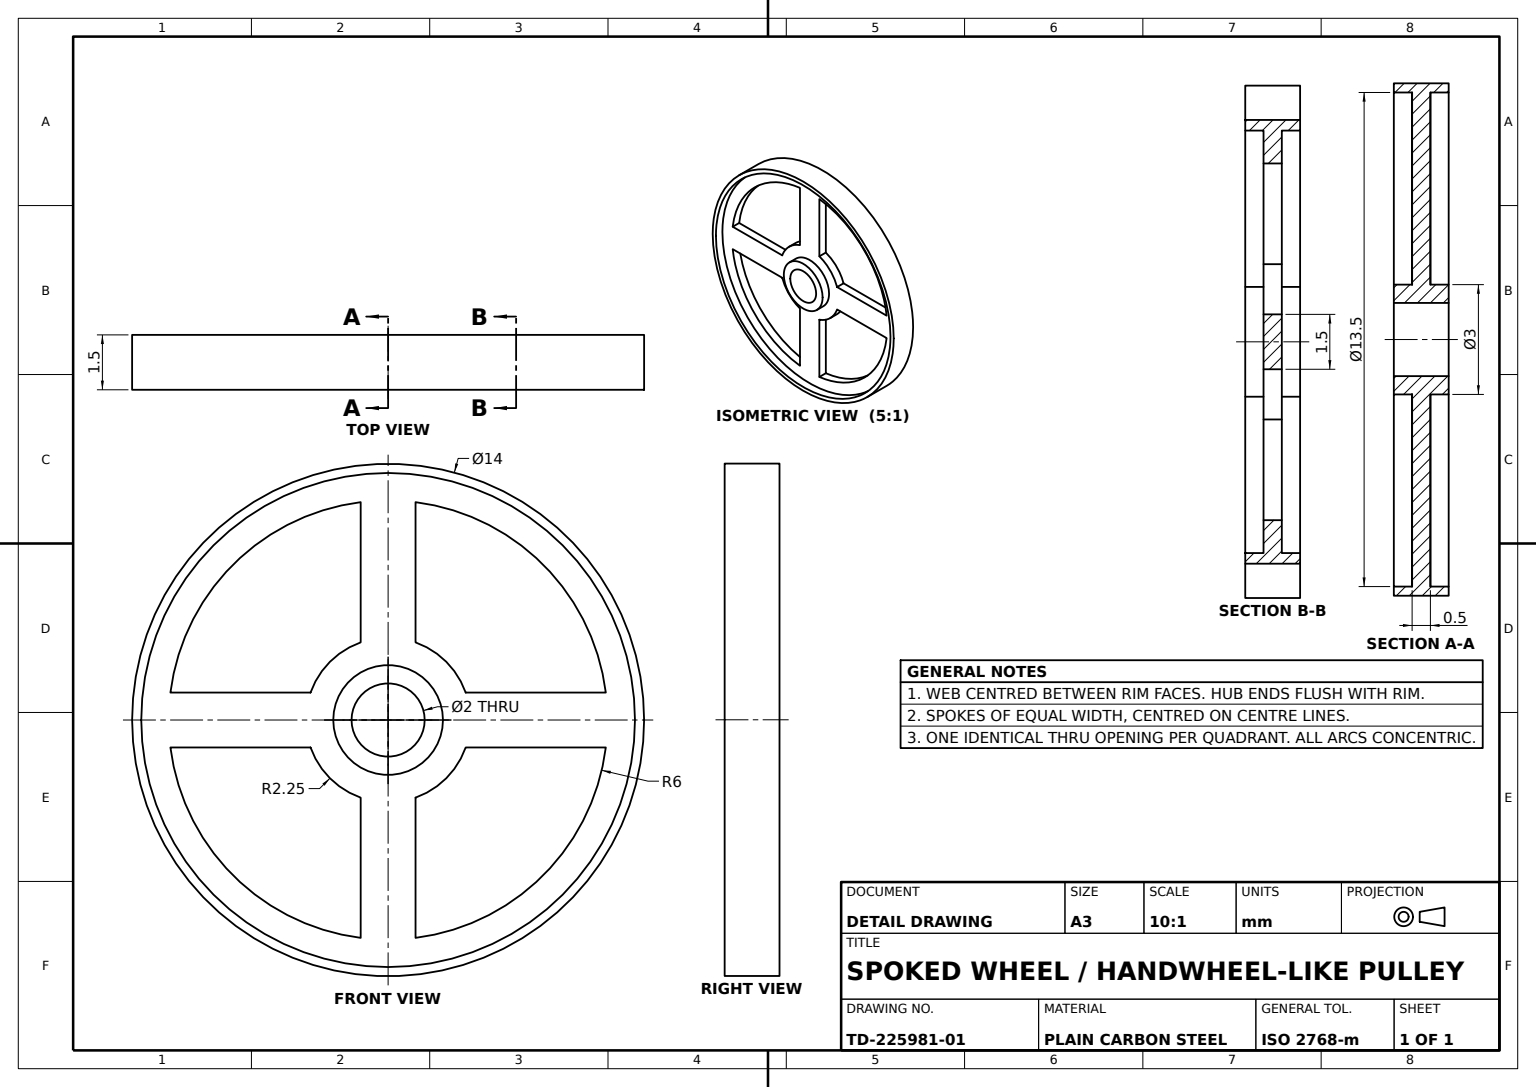
from build123d import *
from build123d.topology import SkipClean

# Parameters (mm, degrees)
HUB_CORE_SKETCH_R           = 2.25
HUB_CORE_DEPTH              = 0.5
HUB_FLANGE_SKETCH_R         = 6
HUB_FLANGE_6_DEPTH          = 0.5
FRONT_HUB_BOSS_SKETCH_R     = 2.25
FRONT_HUB_BOSS_DEPTH        = 0.5
CROSS_START                 = -0.5
CROSS_SLOT_CUT_DEPTH        = 0.5
WEB_START                   = -0.5
WEB_RING_SKETCH_R           = 6.75
WEB_RING_SKETCH_R_2         = 6
WEB_RING_13_5_DEPTH         = 0.5
FRONT_START                 = -0.5
FRONT_HUB_HOLE_SKETCH_R     = 2.25
FRONT_HUB_HOLE_CUT_DEPTH    = 0.5
BACK_HUB_RECESS_SKETCH_R    = 2.25
BACK_HUB_RECESS_CUT_DEPTH   = 0.5
HUB_RING_A_SKETCH_R         = 1.5
HUB_RING_A_DEPTH            = 0.5
HUB_START                   = 0.5
HUB_RING_B_SKETCH_R         = 1.5
HUB_RING_B_DEPTH            = 0.5
SPOKE_1_DEPTH               = 1.5
SPOKE_1_GROOVE_A_DEPTH      = 0.625
SPOKE_1_GROOVE_B_DEPTH      = 0.625
SPOKE_2_DEPTH               = 1.5
SPOKE_3_DEPTH               = 1.5
SPOKE_4_DEPTH               = 1.5
SPOKE_GROOVES_A_DEPTH       = 0.65
SPOKE_GROOVES_B_DEPTH       = 0.65
CROSS_SPOKES_DEPTH          = 1.5
CROSS_SPOKES_2_DEPTH        = 1.5
CROSS_SPOKES_3_DEPTH        = 1.5
CROSS_SPOKES_4_DEPTH        = 1.5
CROSS_SPOKE_GROOVES_A_DEPTH = 0.625
CROSS_SPOKE_GROOVES_B_DEPTH = 0.625
CENTRE_HOLE_SKETCH_R        = 1
CENTRE_HOLE_CUT_DEPTH       = 10
RIM_START                   = -0.5
RIM_RING_1_SKETCH_R         = 7
RIM_RING_1_SKETCH_R_2       = 6.75
RIM_RING_1_14_DEPTH         = 0.5
RIM_RING_2_SKETCH_R         = 7
RIM_RING_2_SKETCH_R_2       = 6.75
RIM_RING_2_14_DEPTH         = 0.5
RIM_START_2                 = 0.5
RIM_RING_3_SKETCH_R         = 7
RIM_RING_3_SKETCH_R_2       = 6.75
RIM_RING_3_14_DEPTH         = 0.5


with BuildPart() as part:
    # Hub Core Sketch → Hub Core (new body)
    with BuildSketch(Plane.XY):
        Circle(HUB_CORE_SKETCH_R)
    extrude(amount=HUB_CORE_DEPTH)

    # Hub Flange Sketch → Hub Flange Ø6 (add)
    with BuildSketch(Plane.XY.offset(0.5)):
        Circle(HUB_FLANGE_SKETCH_R)
    extrude(amount=HUB_FLANGE_6_DEPTH)

    # Front Hub Boss Sketch → Front Hub Boss (add)
    with BuildSketch(Plane.XY.offset(1)):
        Circle(FRONT_HUB_BOSS_SKETCH_R)
    extrude(amount=FRONT_HUB_BOSS_DEPTH)

    # Cross Slot Sketch → Cross Slot Cut (cut)
    with SkipClean():  # the faces are left unmerged after this step: merging them gives an invalid solid
        with BuildSketch(Plane.XY.offset(1).offset(CROSS_START)):
            with BuildLine():
                ThreePointArc((-2.121320344, 0.75), (-1.590990258, 1.590990258), (-0.75, 2.121320344))
                Line((-0.75, 2.121320344), (-0.75, 5.95294045))
                ThreePointArc((-0.75, 5.95294045), (-4.242640687, 4.242640687), (-5.95294045, 0.75))
                Line((-5.95294045, 0.75), (-2.121320344, 0.75))
            make_face()
            with BuildLine():
                Line((0.75, 5.95294045), (0.75, 2.121320344))
                ThreePointArc((0.75, 2.121320344), (1.590990258, 1.590990258), (2.121320344, 0.75))
                Line((2.121320344, 0.75), (5.95294045, 0.75))
                ThreePointArc((5.95294045, 0.75), (4.242640687, 4.242640687), (0.75, 5.95294045))
            make_face()
            with BuildLine():
                ThreePointArc((2.121320344, -0.75), (1.590990258, -1.590990258), (0.75, -2.121320344))
                Line((0.75, -2.121320344), (0.75, -5.95294045))
                ThreePointArc((0.75, -5.95294045), (4.242640687, -4.242640687), (5.95294045, -0.75))
                Line((5.95294045, -0.75), (2.121320344, -0.75))
            make_face()
            with BuildLine():
                Line((-0.75, -5.95294045), (-0.75, -2.121320344))
                ThreePointArc((-0.75, -2.121320344), (-1.590990258, -1.590990258), (-2.121320344, -0.75))
                Line((-2.121320344, -0.75), (-5.95294045, -0.75))
                ThreePointArc((-5.95294045, -0.75), (-4.242640687, -4.242640687), (-0.75, -5.95294045))
            make_face()
        extrude(amount=CROSS_SLOT_CUT_DEPTH, mode=Mode.SUBTRACT)

    # Web Ring Sketch → Web Ring Ø13.5 (add)
    with SkipClean():  # the faces are left unmerged after this step: merging them gives an invalid solid
        with BuildSketch(Plane.XY.offset(1).offset(WEB_START)):
            Circle(WEB_RING_SKETCH_R)
            Circle(WEB_RING_SKETCH_R_2, mode=Mode.SUBTRACT)
        extrude(amount=WEB_RING_13_5_DEPTH)

    # Front Hub Hole Sketch → Front Hub Hole Cut (cut)
    with SkipClean():  # the faces are left unmerged after this step: merging them gives an invalid solid
        with BuildSketch(Plane.XY.offset(1.5).offset(FRONT_START)):
            with Locations(Location((0, 0, 0), (0, 0, 199.471220634))):
                Circle(FRONT_HUB_HOLE_SKETCH_R)
        extrude(amount=FRONT_HUB_HOLE_CUT_DEPTH, mode=Mode.SUBTRACT)

    # Back Hub Recess Sketch → Back Hub Recess Cut (cut)
    with BuildSketch(Plane(origin=(0, 0, 0), x_dir=(-1, 0, 0), z_dir=(0, 0, -1))):
        Circle(BACK_HUB_RECESS_SKETCH_R)
    extrude(amount=-BACK_HUB_RECESS_CUT_DEPTH, mode=Mode.SUBTRACT)

    # Hub Ring A Sketch → Hub Ring A (add)
    with BuildSketch(Plane(origin=(0, 0, 0.5), x_dir=(-1, 0, 0), z_dir=(0, 0, -1))):
        Circle(HUB_RING_A_SKETCH_R)
    extrude(amount=HUB_RING_A_DEPTH)

    # Hub Ring B Sketch → Hub Ring B (add)
    with BuildSketch(Plane.XY.offset(1).offset(HUB_START)):
        with Locations(Location((0, 0, 0), (0, 0, 180))):
            Circle(HUB_RING_B_SKETCH_R)
    extrude(amount=-HUB_RING_B_DEPTH)

    # Centre Hole Sketch → Centre Hole Cut (cut)
    with BuildSketch(Plane.XY.offset(1.5)):
        Circle(CENTRE_HOLE_SKETCH_R)
    extrude(amount=-CENTRE_HOLE_CUT_DEPTH, mode=Mode.SUBTRACT)

    # Rim Ring 1 Sketch → Rim Ring 1 Ø14 (add)
    with BuildSketch(Plane.XY.offset(1).offset(RIM_START)):
        Circle(RIM_RING_1_SKETCH_R)
        Circle(RIM_RING_1_SKETCH_R_2, mode=Mode.SUBTRACT)
    extrude(amount=RIM_RING_1_14_DEPTH)

    # Rim Ring 2 Sketch → Rim Ring 2 Ø14 (add)
    with BuildSketch(Plane.XY.offset(1)):
        Circle(RIM_RING_2_SKETCH_R)
        Circle(RIM_RING_2_SKETCH_R_2, mode=Mode.SUBTRACT)
    extrude(amount=RIM_RING_2_14_DEPTH)

    # Rim Ring 3 Sketch → Rim Ring 3 Ø14 (add)
    with BuildSketch(Plane(origin=(0, 0, 0.5), x_dir=(-1, 0, 0), z_dir=(0, 0, -1)).offset(RIM_START_2)):
        with Locations(Location((0, 0, 0), (0, 0, 180))):
            Circle(RIM_RING_3_SKETCH_R)
        with Locations(Location((0, 0, 0), (0, 0, 180))):
            Circle(RIM_RING_3_SKETCH_R_2, mode=Mode.SUBTRACT)
    extrude(amount=-RIM_RING_3_14_DEPTH)


with BuildPart() as body_2:
    # Spoke 1 Sketch → Spoke 1 (new body)
    with BuildSketch(Plane.XZ.offset(0.75)):
        Polygon((-1.5, 1.5), (-1.5, 1), (-6.75, 1), (-5.25, 1.5), align=None)
    extrude(amount=-SPOKE_1_DEPTH)

    # Spoke 1 Groove A Sketch → Spoke 1 Groove A (cut)
    with BuildSketch(Plane.XZ.offset(0.75)):
        Polygon((-6.75, 1), (-5.25, 1.5), (-1.5, 1.5), (-1.5, 1), align=None)
    extrude(amount=-SPOKE_1_GROOVE_A_DEPTH, mode=Mode.SUBTRACT)

    # Spoke 1 Groove B Sketch → Spoke 1 Groove B (cut)
    with BuildSketch(Plane(origin=(0, 0.75, 0), x_dir=(1, 0, 0), z_dir=(0, 1, 0))):
        Polygon((-1.5, -1.5), (-1.5, -1), (-6.75, -1), (-5.25, -1.5), align=None)
    extrude(amount=-SPOKE_1_GROOVE_B_DEPTH, mode=Mode.SUBTRACT)


with BuildPart() as body_3:
    # Spoke 2 Sketch → Spoke 2 (new body)
    with BuildSketch(Plane.XZ.offset(0.75)):
        Polygon((5.25, 1.5), (1.5, 1.5), (1.5, 1), (2.121320344, 1), (5.95294045, 1), (6.75, 1), align=None)
    extrude(amount=-SPOKE_2_DEPTH)


with BuildPart() as body_4:
    # Spoke 3 Sketch → Spoke 3 (new body)
    with BuildSketch(Plane.XZ.offset(0.75)):
        Polygon((1.5, 0), (1.5, 0.5), (6.75, 0.5), (5.25, 0), align=None)
    extrude(amount=-SPOKE_3_DEPTH)


with BuildPart() as body_5:
    # Spoke 4 Sketch → Spoke 4 (new body)
    with BuildSketch(Plane.XZ.offset(0.75)):
        Polygon((-1.5, 0), (-5.25, 0), (-6.75, 0.5), (-1.5, 0.5), align=None)
    extrude(amount=-SPOKE_4_DEPTH)


with BuildPart() as spoke_grooves_a_tool:
    # Spoke Grooves A Sketch → Spoke Grooves A (new body)
    with BuildSketch(Plane.XZ.offset(0.75)):
        Polygon((1.5, 1.5), (1.5, 1), (6.75, 1), (5.25, 1.5), align=None)
        Polygon((1.5, 0), (1.5, 0.5), (6.75, 0.5), (5.25, 0), align=None)
        Polygon((-6.75, 0.5), (-1.5, 0.5), (-1.5, 0), (-5.25, 0), align=None)
    extrude(amount=-SPOKE_GROOVES_A_DEPTH)


with BuildPart() as body_3_1:
    add(body_3.part)

    # Spoke Grooves A: cut by spoke_grooves_a_tool
    add(spoke_grooves_a_tool.part, mode=Mode.SUBTRACT)


with BuildPart() as body_4_1:
    add(body_4.part)

    # Spoke Grooves A: cut by spoke_grooves_a_tool
    add(spoke_grooves_a_tool.part, mode=Mode.SUBTRACT)


with BuildPart() as body_5_1:
    add(body_5.part)

    # Spoke Grooves A: cut by spoke_grooves_a_tool
    add(spoke_grooves_a_tool.part, mode=Mode.SUBTRACT)


with BuildPart() as spoke_grooves_b_tool:
    # Spoke Grooves B Sketch → Spoke Grooves B (new body)
    with BuildSketch(Plane(origin=(0, 0.75, 0), x_dir=(1, 0, 0), z_dir=(0, 1, 0))):
        Polygon((1.5, 0), (5.25, 0), (6.75, -0.5), (1.5, -0.5), align=None)
        Polygon((1.5, -1.5), (1.5, -1), (6.75, -1), (5.25, -1.5), align=None)
        Polygon((-6.75, -0.5), (-1.5, -0.5), (-1.5, 0), (-5.25, 0), align=None)
    extrude(amount=-SPOKE_GROOVES_B_DEPTH)


with BuildPart() as body_3_2:
    add(body_3_1.part)

    # Spoke Grooves B: cut by spoke_grooves_b_tool
    add(spoke_grooves_b_tool.part, mode=Mode.SUBTRACT)


with BuildPart() as body_4_2:
    add(body_4_1.part)

    # Spoke Grooves B: cut by spoke_grooves_b_tool
    add(spoke_grooves_b_tool.part, mode=Mode.SUBTRACT)


with BuildPart() as body_5_2:
    add(body_5_1.part)

    # Spoke Grooves B: cut by spoke_grooves_b_tool
    add(spoke_grooves_b_tool.part, mode=Mode.SUBTRACT)


with BuildPart() as body_6:
    # Cross Spokes Sketch → Cross Spokes (new body)
    with BuildSketch(Plane.ZY.offset(0.75)):
        Polygon((1, 1.5), (1, 6.75), (1.5, 5.25), (1.5, 1.5), align=None)
    extrude(amount=-CROSS_SPOKES_DEPTH)


with BuildPart() as body_7:
    # Cross Spokes Sketch → Cross Spokes 2 (new body)
    with BuildSketch(Plane.ZY.offset(0.75)):
        Polygon((0.5, 1.5), (0.5, 6.75), (0, 5.25), (0, 1.5), align=None)
    extrude(amount=-CROSS_SPOKES_2_DEPTH)


with BuildPart() as body_8:
    # Cross Spokes Sketch → Cross Spokes 3 (new body)
    with BuildSketch(Plane.ZY.offset(0.75)):
        Polygon((1, -1.5), (1, -6.75), (1.5, -5.25), (1.5, -1.5), align=None)
    extrude(amount=-CROSS_SPOKES_3_DEPTH)


with BuildPart() as body_9:
    # Cross Spokes Sketch → Cross Spokes 4 (new body)
    with BuildSketch(Plane.ZY.offset(0.75)):
        Polygon((0.5, -1.5), (0.5, -6.75), (0, -5.25), (0, -1.5), align=None)
    extrude(amount=-CROSS_SPOKES_4_DEPTH)


with BuildPart() as cross_spoke_grooves_a_tool:
    # Cross Spoke Grooves A Sketch → Cross Spoke Grooves A (new body)
    with BuildSketch(Plane.ZY.offset(0.75)):
        Polygon((1.5, 1.5), (1, 1.5), (1, 6.75), (1.5, 5.25), align=None)
        Polygon((0.5, 6.75), (0.5, 1.5), (0, 1.5), (0, 5.25), align=None)
        Polygon((1, -6.75), (1, -1.5), (1.5, -1.5), (1.5, -5.25), align=None)
        Polygon((0, -1.5), (0.5, -1.5), (0.5, -6.75), (0, -5.25), align=None)
    extrude(amount=-CROSS_SPOKE_GROOVES_A_DEPTH)


with BuildPart() as body_6_1:
    add(body_6.part)

    # Cross Spoke Grooves A: cut by cross_spoke_grooves_a_tool
    add(cross_spoke_grooves_a_tool.part, mode=Mode.SUBTRACT)


with BuildPart() as body_7_1:
    add(body_7.part)

    # Cross Spoke Grooves A: cut by cross_spoke_grooves_a_tool
    add(cross_spoke_grooves_a_tool.part, mode=Mode.SUBTRACT)


with BuildPart() as body_8_1:
    add(body_8.part)

    # Cross Spoke Grooves A: cut by cross_spoke_grooves_a_tool
    add(cross_spoke_grooves_a_tool.part, mode=Mode.SUBTRACT)


with BuildPart() as body_9_1:
    add(body_9.part)

    # Cross Spoke Grooves A: cut by cross_spoke_grooves_a_tool
    add(cross_spoke_grooves_a_tool.part, mode=Mode.SUBTRACT)


with BuildPart() as cross_spoke_grooves_b_tool:
    # Cross Spoke Grooves B Sketch → Cross Spoke Grooves B (new body)
    with BuildSketch(Plane(origin=(0.75, 0, 0), x_dir=(0, 0, -1), z_dir=(1, 0, 0))):
        Polygon((0, 1.5), (-0.5, 1.5), (-0.5, 6.75), (0, 5.25), align=None)
        Polygon((-1, 6.75), (-1, 1.5), (-1.5, 1.5), (-1.5, 5.25), align=None)
        Polygon((0, -1.5), (0, -5.25), (-0.5, -6.75), (-0.5, -1.5), align=None)
        Polygon((-1.5, -1.5), (-1.5, -5.25), (-1, -6.75), (-1, -1.5), align=None)
    extrude(amount=-CROSS_SPOKE_GROOVES_B_DEPTH)


with BuildPart() as body_6_2:
    add(body_6_1.part)

    # Cross Spoke Grooves B: cut by cross_spoke_grooves_b_tool
    add(cross_spoke_grooves_b_tool.part, mode=Mode.SUBTRACT)


with BuildPart() as body_7_2:
    add(body_7_1.part)

    # Cross Spoke Grooves B: cut by cross_spoke_grooves_b_tool
    add(cross_spoke_grooves_b_tool.part, mode=Mode.SUBTRACT)


with BuildPart() as body_8_2:
    add(body_8_1.part)

    # Cross Spoke Grooves B: cut by cross_spoke_grooves_b_tool
    add(cross_spoke_grooves_b_tool.part, mode=Mode.SUBTRACT)


with BuildPart() as body_9_2:
    add(body_9_1.part)

    # Cross Spoke Grooves B: cut by cross_spoke_grooves_b_tool
    add(cross_spoke_grooves_b_tool.part, mode=Mode.SUBTRACT)


solid = part.part
